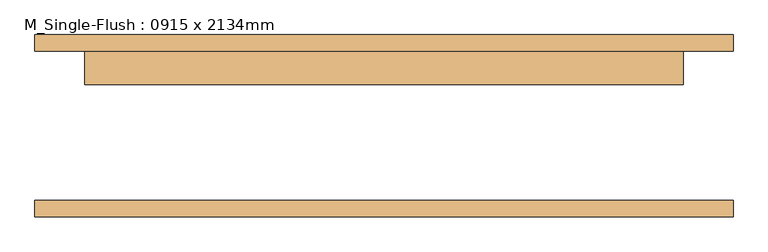
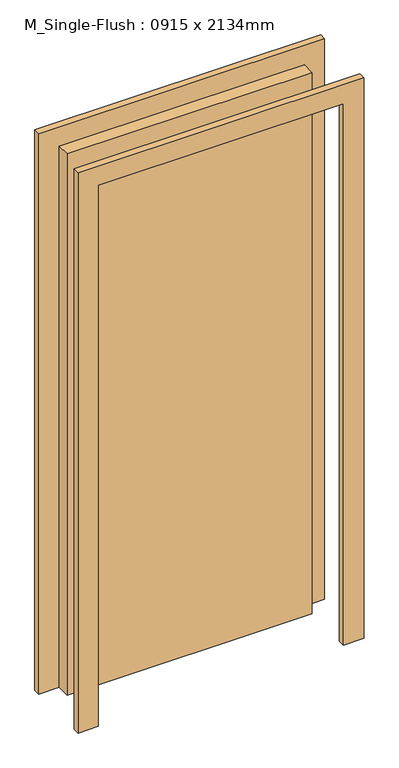
"""IFC4 building model written with IfcOpenShell, lengths in millimetres: door geometry, M_Single-Flush : 0915 x 2134mm."""

from ifc_helpers import new_model, si_unit, frame, origin, origin_with_axes, place, context, project, spatial, polyline, outline, extrude, source, transform, mapped, element, save


def m_single_flush_0915_x_2134mm_1ddf3370(model_context):
    return source(origin(), model_context, "Body", "SweptSolid", [
        extrude(outline(polyline([(2210.0, -533.5), (0.0, -533.5), (0.0, -457.5), (2134.0, -457.5), (2134.0, 457.5), (0.0, 457.5), (0.0, 533.5), (2210.0, 533.5), (2210.0, -533.5)])), frame((0.0, 114.3, 0.0), z_axis=(0.0, 1.0, 0.0), x_axis=(0.0, 0.0, 1.0)), (0.0, 0.0, 1.0), 25.0),
        extrude(outline(polyline([(2210.0, 533.5), (2210.0, -533.5), (0.0, -533.5), (0.0, -457.5), (2134.0, -457.5), (2134.0, 457.5), (0.0, 457.5), (0.0, 533.5), (2210.0, 533.5)])), frame((0.0, -139.3, 0.0), z_axis=(0.0, 1.0, 0.0), x_axis=(0.0, 0.0, 1.0)), (0.0, 0.0, 1.0), 25.0),
        extrude(outline(polyline([(457.5, 63.3), (-457.5, 63.3), (-457.5, 114.3), (457.5, 114.3), (457.5, 63.3)])), origin_with_axes(), (0.0, 0.0, 1.0), 2134.0),
    ])


if __name__ == "__main__":
    model = new_model("IFC4")
    model_context = context("Model", 3, world=origin())
    ifc_project = project(units=[si_unit("LENGTHUNIT", "METRE", prefix="MILLI")], contexts=[model_context])
    site = spatial("IfcSite", under=ifc_project)
    building = spatial("IfcBuilding", under=site)
    placement = place(None, origin())
    m_single_flush_0915_x_2134mm_shape = m_single_flush_0915_x_2134mm_1ddf3370(model_context)
    element("IfcDoor", 1, ObjectType="M_Single-Flush : 0915 x 2134mm", at=placement, inside=building, context=model_context, shape_type="MappedRepresentation", body=[
        mapped(m_single_flush_0915_x_2134mm_shape, transform((0.0, 0.0, 0.0), x_axis=(1.0, 0.0, 0.0), y_axis=(0.0, 1.0, 0.0), z_axis=(0.0, 0.0, 1.0))),
    ])
    save(model, "model.ifc")

# Revit data of these elements
# Type "M_Single-Flush : 0915 x 2134mm"
#   Type Mark = "15"
#   Thickness = 51 mm
#   Height = 2134 mm
#   Trim Projection Ext = 25 mm
#   Trim Projection Int = 25 mm
#   Trim Width = 76 mm
#   Width = 915 mm
#   Door Material = Door - Panel
#   Frame Material = Door - Frame
#   Function = (empty or 0)
#   Wall Closure = (empty or 0)
# Element 1 (IfcDoor, "M_Single-Flush : 0915 x 2134mm")
#   Materials on its faces: "Door - Frame", "Door - Panel"
# Materials
#   "Door - Panel": class "Wood", colour RGB 114 82 51, transparency 0
#   "Door - Frame": colour RGB 153 76 43, transparency 0
